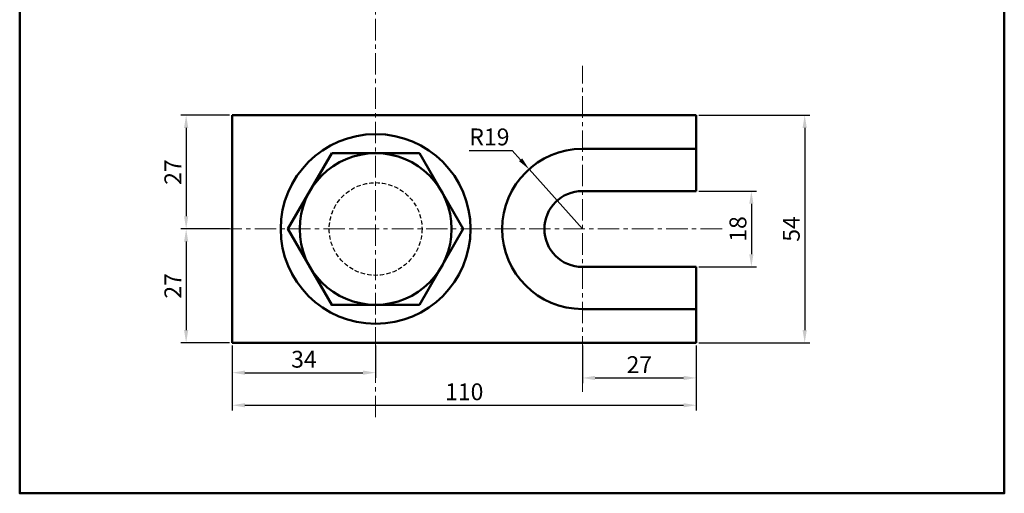
# Model space of a CAD drawing. Units: millimetres. Extents: x 458 to 691, y 231 to 528.
# Tile 1 of 2: x 458 to 691, y 231 to 343. Entities that reach past the tile are written whole.
import ezdxf

# ---------------------------------------------------------------- set-up
doc = ezdxf.new("R2010")
doc.units = ezdxf.units.MM
doc.header["$LTSCALE"] = 0.4
doc.linetypes.add('CENTER', pattern=[50.8, 31.75, -6.35, 6.35, -6.35])
doc.linetypes.add('HIDDEN', pattern=[9.525, 6.35, -3.175])
for name, color, linetype, lineweight in [('M-CNTR', 1, 'CENTER', 18), ('M-DIMS', 2, 'Continuous', 25), ('M-HIDN', 4, 'HIDDEN', 25), ('M-OUTL', 7, 'Continuous', 50)]:
    doc.layers.add(name, color=color, linetype=linetype, lineweight=lineweight)
doc.styles.get("Standard").update_dxf_attribs({"font": 'arial.ttf'})
doc.dimstyles.new('ISO-25', dxfattribs={"dimtxt": 4, "dimasz": 3, "dimexe": 1.25, "dimexo": 0.625, "dimtad": 1, "dimtoh": 1, "dimtxsty": 'Standard', "dimcen": 2.5, "dimadec": 0, "dimazin": 0, "dimtfac": 1, "dimtmove": 0, "dimatfit": 3, "dimfxl": 1, "dimarcsym": 0})

# ---------------------------------------------------------------- blocks, each defined once
blk = doc.blocks.new('*D25')
at = {"layer": 'Defpoints', "color": 0, "ltscale": 0.4, "transparency": 16777216}
for p in [(508.27, 320.39), (497.36, 293.39), (508.27, 293.39)]:
    blk.add_point(p, dxfattribs=at)
at = {"layer": 'M-DIMS', "color": 0, "lineweight": -2, "ltscale": 0.4, "transparency": 16777216}
for p, q in [((507.65, 320.39), (496.11, 320.39)), ((497.36, 317.39), (497.36, 296.39)), ((507.65, 293.39), (496.11, 293.39))]:
    blk.add_line(p, q, dxfattribs=at)
at = {"layer": 'M-DIMS', "color": 0, "ltscale": 0.4, "transparency": 16777216}
for points in [[(496.86, 317.39), (497.86, 317.39), (497.36, 320.39)], [(496.86, 296.39), (497.86, 296.39), (497.36, 293.39)]]:
    blk.add_solid(points, dxfattribs=at)
at = {"layer": 'M-DIMS', "color": 0, "ltscale": 0.4, "transparency": 16777216, "insert": (494.73, 306.89), "char_height": 4, "attachment_point": 5, "rotation": 90}
blk.add_mtext('27', dxfattribs=at)
blk = doc.blocks.new('*D26')
at = {"layer": 'Defpoints', "color": 0, "ltscale": 0.4, "transparency": 16777216}
for p in [(508.27, 293.39), (497.36, 266.39), (508.27, 266.39)]:
    blk.add_point(p, dxfattribs=at)
at = {"layer": 'M-DIMS', "color": 0, "lineweight": -2, "ltscale": 0.4, "transparency": 16777216}
for p, q in [((507.65, 293.39), (496.11, 293.39)), ((497.36, 290.39), (497.36, 269.39)), ((507.65, 266.39), (496.11, 266.39))]:
    blk.add_line(p, q, dxfattribs=at)
at = {"layer": 'M-DIMS', "color": 0, "ltscale": 0.4, "transparency": 16777216}
for points in [[(496.86, 290.39), (497.86, 290.39), (497.36, 293.39)], [(496.86, 269.39), (497.86, 269.39), (497.36, 266.39)]]:
    blk.add_solid(points, dxfattribs=at)
at = {"layer": 'M-DIMS', "color": 0, "ltscale": 0.4, "transparency": 16777216, "insert": (494.73, 279.89), "char_height": 4, "attachment_point": 5, "rotation": 90}
blk.add_mtext('27', dxfattribs=at)
blk = doc.blocks.new('*D27')
at = {"layer": 'Defpoints', "color": 0, "ltscale": 0.4, "transparency": 16777216}
for p in [(508.27, 266.39), (542.27, 266.39), (542.27, 259.29)]:
    blk.add_point(p, dxfattribs=at)
at = {"layer": 'M-DIMS', "color": 0, "lineweight": -2, "ltscale": 0.4, "transparency": 16777216}
for p, q in [((508.27, 265.76), (508.27, 258.04)), ((542.27, 265.76), (542.27, 258.04)), ((511.27, 259.29), (539.27, 259.29))]:
    blk.add_line(p, q, dxfattribs=at)
at = {"layer": 'M-DIMS', "color": 0, "ltscale": 0.4, "transparency": 16777216}
for points in [[(511.27, 259.79), (511.27, 258.79), (508.27, 259.29)], [(539.27, 259.79), (539.27, 258.79), (542.27, 259.29)]]:
    blk.add_solid(points, dxfattribs=at)
at = {"layer": 'M-DIMS', "color": 0, "ltscale": 0.4, "transparency": 16777216, "insert": (525.27, 261.96), "char_height": 4, "attachment_point": 5}
blk.add_mtext('34', dxfattribs=at)
blk = doc.blocks.new('*D28')
at = {"layer": 'Defpoints', "color": 0, "ltscale": 0.4, "transparency": 16777216}
for p in [(508.27, 266.39), (618.27, 266.39), (618.27, 251.56)]:
    blk.add_point(p, dxfattribs=at)
at = {"layer": 'M-DIMS', "color": 0, "lineweight": -2, "ltscale": 0.4, "transparency": 16777216}
for p, q in [((508.27, 265.76), (508.27, 250.31)), ((618.27, 265.76), (618.27, 250.31)), ((511.27, 251.56), (615.27, 251.56))]:
    blk.add_line(p, q, dxfattribs=at)
at = {"layer": 'M-DIMS', "color": 0, "ltscale": 0.4, "transparency": 16777216}
for points in [[(511.27, 252.06), (511.27, 251.06), (508.27, 251.56)], [(615.27, 252.06), (615.27, 251.06), (618.27, 251.56)]]:
    blk.add_solid(points, dxfattribs=at)
at = {"layer": 'M-DIMS', "color": 0, "ltscale": 0.4, "transparency": 16777216, "insert": (563.27, 254.23), "char_height": 4, "attachment_point": 5}
blk.add_mtext('110', dxfattribs=at)
blk = doc.blocks.new('*D29')
at = {"layer": 'Defpoints', "color": 0, "ltscale": 0.4, "transparency": 16777216}
for p in [(618.27, 302.39), (618.27, 284.39), (631.32, 284.39)]:
    blk.add_point(p, dxfattribs=at)
at = {"layer": 'M-DIMS', "color": 0, "lineweight": -2, "ltscale": 0.4, "transparency": 16777216}
for p, q in [((618.9, 302.39), (632.57, 302.39)), ((631.32, 299.39), (631.32, 287.39)), ((618.9, 284.39), (632.57, 284.39))]:
    blk.add_line(p, q, dxfattribs=at)
at = {"layer": 'M-DIMS', "color": 0, "ltscale": 0.4, "transparency": 16777216}
for points in [[(630.82, 299.39), (631.82, 299.39), (631.32, 302.39)], [(630.82, 287.39), (631.82, 287.39), (631.32, 284.39)]]:
    blk.add_solid(points, dxfattribs=at)
at = {"layer": 'M-DIMS', "color": 0, "ltscale": 0.4, "transparency": 16777216, "insert": (628.66, 293.39), "char_height": 4, "attachment_point": 5, "rotation": 90}
blk.add_mtext('18', dxfattribs=at)
blk = doc.blocks.new('*D30')
at = {"layer": 'Defpoints', "color": 0, "ltscale": 0.4, "transparency": 16777216}
for p in [(591.27, 266.39), (618.27, 266.39), (618.27, 258.04)]:
    blk.add_point(p, dxfattribs=at)
at = {"layer": 'M-DIMS', "color": 0, "lineweight": -2, "ltscale": 0.4, "transparency": 16777216}
for p, q in [((591.27, 265.76), (591.27, 256.79)), ((618.27, 265.76), (618.27, 256.79)), ((594.27, 258.04), (615.27, 258.04))]:
    blk.add_line(p, q, dxfattribs=at)
at = {"layer": 'M-DIMS', "color": 0, "ltscale": 0.4, "transparency": 16777216}
for points in [[(594.27, 258.54), (594.27, 257.54), (591.27, 258.04)], [(615.27, 258.54), (615.27, 257.54), (618.27, 258.04)]]:
    blk.add_solid(points, dxfattribs=at)
at = {"layer": 'M-DIMS', "color": 0, "ltscale": 0.4, "transparency": 16777216, "insert": (604.77, 260.68), "char_height": 4, "attachment_point": 5}
blk.add_mtext('27', dxfattribs=at)
blk = doc.blocks.new('*D31')
at = {"layer": 'Defpoints', "color": 0, "ltscale": 0.4, "transparency": 16777216}
for p in [(618.27, 320.39), (618.27, 266.39), (643.96, 266.39)]:
    blk.add_point(p, dxfattribs=at)
at = {"layer": 'M-DIMS', "color": 0, "lineweight": -2, "ltscale": 0.4, "transparency": 16777216}
for p, q in [((618.9, 320.39), (645.21, 320.39)), ((643.96, 317.39), (643.96, 269.39)), ((618.9, 266.39), (645.21, 266.39))]:
    blk.add_line(p, q, dxfattribs=at)
at = {"layer": 'M-DIMS', "color": 0, "ltscale": 0.4, "transparency": 16777216}
for points in [[(643.46, 317.39), (644.46, 317.39), (643.96, 320.39)], [(643.46, 269.39), (644.46, 269.39), (643.96, 266.39)]]:
    blk.add_solid(points, dxfattribs=at)
at = {"layer": 'M-DIMS', "color": 0, "ltscale": 0.4, "transparency": 16777216, "insert": (641.3, 293.39), "char_height": 4, "attachment_point": 5, "rotation": 90}
blk.add_mtext('54', dxfattribs=at)
blk = doc.blocks.new('*D32')
at = {"layer": 'Defpoints', "color": 0, "ltscale": 0.4, "transparency": 16777216}
for p in [(578.63, 307.57), (591.27, 293.39)]:
    blk.add_point(p, dxfattribs=at)
at = {"layer": 'M-DIMS', "color": 0, "lineweight": -2, "ltscale": 0.4, "transparency": 16777216}
for p, q in [((564.45, 312.05), (574.64, 312.05)), ((574.64, 312.05), (576.63, 309.81)), ((591.27, 293.39), (578.63, 307.57))]:
    blk.add_line(p, q, dxfattribs=at)
at = {"layer": 'M-DIMS', "color": 0, "ltscale": 0.4, "transparency": 16777216}
blk.add_solid([(577.01, 310.14), (576.26, 309.48), (578.63, 307.57)], dxfattribs=at)
at = {"layer": 'M-DIMS', "color": 0, "ltscale": 0.4, "transparency": 16777216, "insert": (569.23, 314.72), "char_height": 4, "attachment_point": 5}
blk.add_mtext('R19', dxfattribs=at)

msp = doc.modelspace()

# ---------------------------------------------------------------- linework, layer by layer
at = {"layer": 'M-CNTR', "ltscale": 0.4}
for p, q in [((542.271, 248.744), (542.271, 482.881)), ((591.271, 254.766), (591.271, 332.096)), ((497.363, 293.387), (624.903, 293.387))]:
    msp.add_line(p, q, dxfattribs=at)
at = {"layer": 'M-HIDN', "ltscale": 0.4}
msp.add_circle((542.271, 293.387), 11, dxfattribs=at)
at = {"layer": 'M-OUTL', "ltscale": 0.4}
for p, q in [((508.271, 320.387), (508.271, 266.387)), ((618.271, 320.387), (508.271, 320.387)), ((618.271, 302.387), (618.271, 320.387)), ((591.271, 312.387), (618.271, 312.387)), ((591.271, 302.387), (618.271, 302.387)), ((591.271, 284.387), (618.271, 284.387)), ((618.271, 266.387), (618.271, 284.387)), ((591.271, 274.387), (618.271, 274.387)), ((508.271, 266.387), (618.271, 266.387))]:
    msp.add_line(p, q, dxfattribs=at)
for points in [[(457.908, 527.656), (691.271, 527.656), (691.271, 230.656), (457.908, 230.656)], [(531.878, 311.387), (521.486, 293.387), (531.878, 275.387), (552.663, 275.387), (563.055, 293.387), (552.663, 311.387)]]:
    msp.add_lwpolyline(points, close=True, dxfattribs=at)
for radius in [22.5, 18]:
    msp.add_circle((542.271, 293.387), radius, dxfattribs=at)
for radius in [19, 9]:
    msp.add_arc((591.271, 293.387), radius, 90, 270, dxfattribs=at)

# ---------------------------------------------------------------- dimensions: what is measured, and where the dimension line sits
at = {"layer": 'M-DIMS', "ltscale": 0.4}
for base, p1, p2, picture, middle in [((497.363, 293.387), (508.271, 320.387), (508.271, 293.387), '*D25', (494.729, 306.887)), ((643.957, 266.387), (618.271, 320.387), (618.271, 266.387), '*D31', (641.298, 293.387)), ((631.323, 284.387), (618.271, 302.387), (618.271, 284.387), '*D29', (628.655, 293.387)), ((497.363, 266.387), (508.271, 293.387), (508.271, 266.387), '*D26', (494.729, 279.887))]:
    dim = msp.add_linear_dim(base=base, p1=p1, p2=p2, angle=90, dimstyle='ISO-25', override={"dimclrd": 0, "dimclre": 0, "dimclrt": 0}, dxfattribs=at)
    dim.commit()
    dim.dimension.update_dxf_attribs({"geometry": picture, "text_midpoint": middle})
dim = msp.add_radius_dim(center=(591.271, 293.387), mpoint=(578.629, 307.571), dimstyle='ISO-25', override={"dimclrd": 0, "dimclre": 0, "dimclrt": 0}, dxfattribs=at)
dim.commit()
dim.dimension.update_dxf_attribs({"geometry": '*D32', "text_midpoint": (569.229, 314.718)})
for base, p1, p2, picture, middle in [((542.271, 259.292), (508.271, 266.387), (542.271, 266.387), '*D27', (525.271, 261.961)), ((618.271, 251.564), (508.271, 266.387), (618.271, 266.387), '*D28', (563.271, 254.231)), ((618.271, 258.042), (591.271, 266.387), (618.271, 266.387), '*D30', (604.771, 260.675))]:
    dim = msp.add_linear_dim(base=base, p1=p1, p2=p2, dimstyle='ISO-25', override={"dimclrd": 0, "dimclre": 0, "dimclrt": 0}, dxfattribs=at)
    dim.commit()
    dim.dimension.update_dxf_attribs({"geometry": picture, "text_midpoint": middle})

doc.saveas('drawing.dxf')
